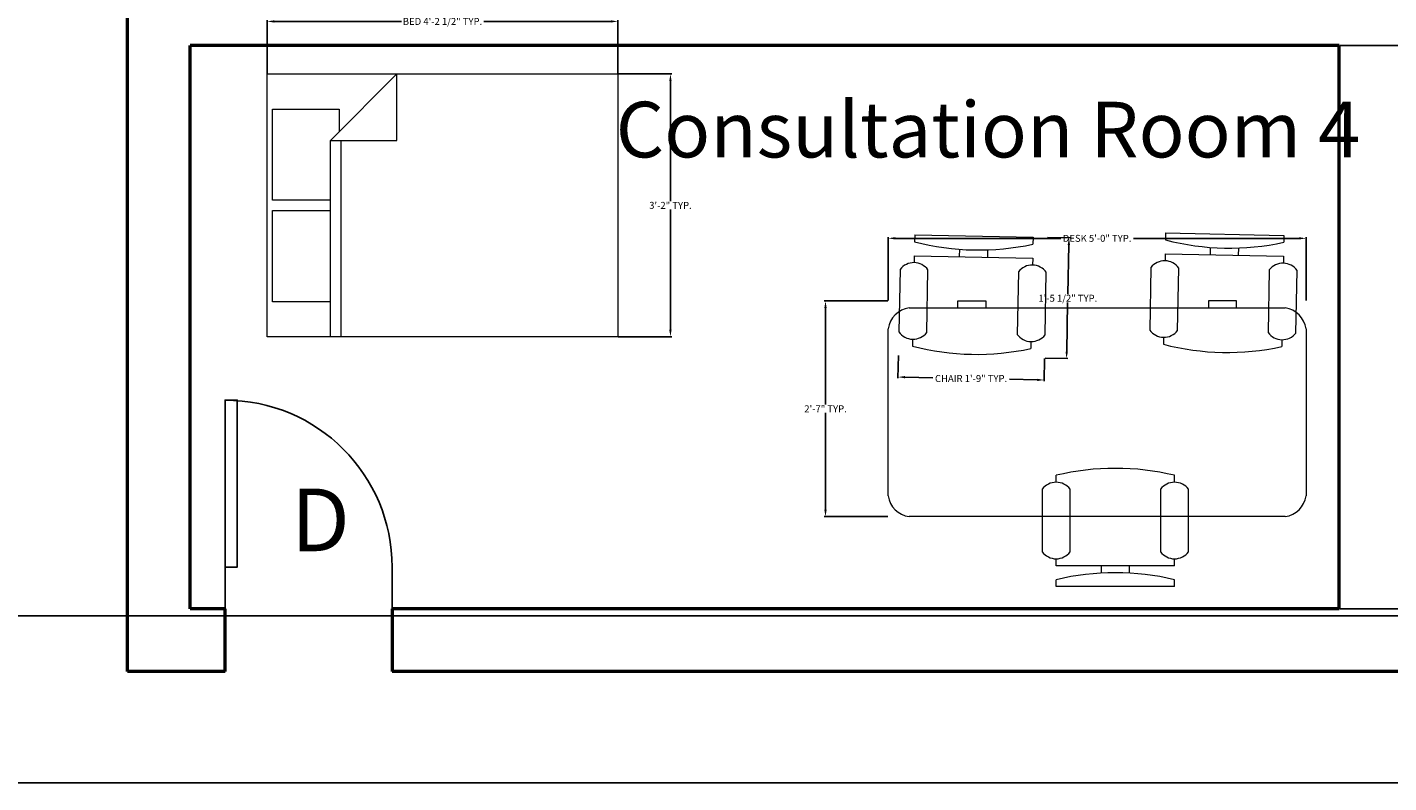
# Model space of a CAD drawing. Units: inches. Extents: x -364 to 705, y -52 to 1250.
# Tile 28 of 34: x 170 to 366, y 806 to 915. Entities that reach past the tile are written whole.
import ezdxf

# ---------------------------------------------------------------- set-up
doc = ezdxf.new("R2010")
doc.units = ezdxf.units.IN
doc.header["$MEASUREMENT"] = 0
for name, color, linetype, lineweight in [('A-ANNO-DIMS', 4, 'Continuous', 18), ('A-ANNO-IDEN', 1, 'Continuous', 18), ('A-AREA-IDEN', 3, 'Continuous', 18), ('A-DOOR', 1, 'Continuous', 25), ('A-FURN', 8, 'Continuous', 18), ('A-WALL', 41, 'Continuous', 50)]:
    doc.layers.add(name, color=color, linetype=linetype, lineweight=lineweight)
doc.styles.get("Standard").update_dxf_attribs({"font": 'arial.ttf'})
doc.dimstyles.get("Standard").update_dxf_attribs({"dimtxt": 1, "dimasz": 1, "dimexe": 0.18, "dimexo": 0.0625, "dimgap": 0.09, "dimtad": 0, "dimtih": 1, "dimtoh": 1, "dimdec": 0, "dimzin": 0, "dimdsep": 46, "dimlunit": 3, "dimtxsty": 'Standard', "dimcen": 0.09, "dimadec": 0, "dimazin": 0, "dimtfac": 1, "dimtdec": 0, "dimtofl": 0, "dimtmove": 0, "dimatfit": 3, "dimfxl": 1, "dimtolj": 1, "dimtzin": 0, "dimarcsym": 0})

# ---------------------------------------------------------------- blocks, each defined once
blk = doc.blocks.new('Chair - Desk')
for p, q in [((-8.5, 0), (-8.5, -1)), ((-8.5, 0), (8.5, 0)), ((8.5, 0), (8.5, -1)), ((-2, -3), (-2, -1.9355)), ((-8.5, -3), (-8.5, -4)), ((-8.5, -3), (8.5, -3)), ((2, -1.9576), (2, -3)), ((8.5, -3), (8.5, -4)), ((-10.5, -5), (-10.5, -14)), ((-6.5, -14), (-6.5, -5)), ((6.5, -5), (6.5, -14)), ((10.5, -14), (10.5, -5)), ((-8.5, -15), (-8.5, -16)), ((8.5, -15), (8.5, -16))]:
    blk.add_line(p, q)
for centre, radius, start, end in [((0, 34.625), 36.625, 256.5803, 283.4197), ((-8.5, -6.5), 2.5, 36.8699, 143.1301), ((8.5, -6.5), 2.5, 36.8699, 143.1301), ((-8.5, -12.5), 2.5, 216.8699, 323.1301), ((8.5, -12.5), 2.5, 216.8699, 323.1301), ((0, 19.625), 36.625, 256.5803, 283.4197)]:
    blk.add_arc(centre, radius, start, end)
blk = doc.blocks.new('Desk - 30 x 60 in.')
for p, q in [((-26.999995, 0), (26.999995, 0)), ((-29.999995, -27), (-29.999995, -3)), ((29.999995, -3), (29.999995, -27)), ((26.999995, -30), (-26.999995, -30)), ((-20.000005, -30), (-20.000005, -31)), ((-20.000005, -31), (-16.000005, -31)), ((-16.000005, -31), (-16.000005, -30)), ((15.999995, -31), (15.999995, -30)), ((19.999995, -31), (15.999995, -31)), ((19.999995, -30), (19.999995, -31))]:
    blk.add_line(p, q)
for centre, start, end in [((-26.499995, -3.5), 98.1301, 171.8699), ((26.499995, -3.5), 8.130102, 81.8699), ((-26.499995, -26.5), 188.1301, 261.8699), ((26.499995, -26.5), 278.1301, 351.8699)]:
    blk.add_arc(centre, 3.535534, start, end)
blk = doc.blocks.new('Bed - Queen')
for p, q in [((0, -80.00003), (0, 0)), ((0, 0), (59.99999, 0)), ((59.99999, 0), (59.99999, -80.00003)), ((7.99999, -1.2), (28.79998, -1.2)), ((7.99999, -14.4), (7.99999, -1.2)), ((28.79998, -1.2), (28.79998, -14.4)), ((31.19999, -1.2), (51.99999, -1.2)), ((31.19999, -14.4), (31.19999, -1.2)), ((51.99999, -1.2), (51.99999, -16.4)), ((0, -14.4), (44.8, -14.4)), ((59.99999, -29.6), (44.8, -14.4)), ((44.8, -14.4), (44.8, -29.6)), ((44.8, -16.8), (0, -16.8)), ((51.99999, -16.4), (46.79936, -16.4)), ((44.8, -29.6), (59.99999, -29.6)), ((59.99999, -80.00003), (0, -80.00003))]:
    blk.add_line(p, q)
blk = doc.blocks.new('*U12')
for p, q in [((0, 0), (0, -6)), ((24, 0), (24, -6))]:
    blk.add_line(p, q)
blk.add_lwpolyline([(0, 0), (0, 24), (1.75, 24), (1.75, 0)], close=True)
blk.add_arc((0, 0), 24, 0, 90)
blk = doc.blocks.new('*D36')
at = {"layer": 'A-ANNO-DIMS', "color": 0, "lineweight": -2, "transparency": 16777216}
for p, q in [((295.27, 867.52), (295.21, 864.25)), ((316.27, 867.09), (316.2, 863.83)), ((296.21, 864.41), (300.21, 864.33)), ((315.21, 864.03), (311.21, 864.11))]:
    blk.add_line(p, q, dxfattribs=at)
at = {"layer": 'A-ANNO-DIMS', "color": 0, "transparency": 16777216}
for points in [[(296.21, 864.58), (296.21, 864.25), (295.21, 864.43)], [(315.21, 864.19), (315.2, 863.86), (316.21, 864.01)]]:
    blk.add_solid(points, dxfattribs=at)
at = {"layer": 'Defpoints', "color": 0, "transparency": 16777216}
for p in [(295.28, 867.58), (316.27, 867.16), (316.21, 864.01)]:
    blk.add_point(p, dxfattribs=at)
at = {"layer": 'A-ANNO-DIMS', "color": 0, "transparency": 16777216, "insert": (305.71, 864.22), "char_height": 1, "attachment_point": 5}
blk.add_mtext('\\A1;CHAIR 1\'-9" TYP.', dxfattribs=at)
blk = doc.blocks.new('*D37')
at = {"layer": 'A-ANNO-DIMS', "color": 0, "lineweight": -2, "transparency": 16777216}
for p, q in [((316.68, 884.49), (319.95, 884.42)), ((319.75, 883.42), (319.61, 876.36)), ((319.44, 868.09), (319.58, 875.15)), ((316.33, 867.16), (319.6, 867.09))]:
    blk.add_line(p, q, dxfattribs=at)
at = {"layer": 'A-ANNO-DIMS', "color": 0, "transparency": 16777216}
for points in [[(319.58, 883.43), (319.92, 883.42), (319.77, 884.42)], [(319.27, 868.1), (319.61, 868.09), (319.42, 867.09)]]:
    blk.add_solid(points, dxfattribs=at)
at = {"layer": 'Defpoints', "color": 0, "transparency": 16777216}
for p in [(316.62, 884.49), (319.77, 884.42), (316.27, 867.16)]:
    blk.add_point(p, dxfattribs=at)
at = {"layer": 'A-ANNO-DIMS', "color": 0, "transparency": 16777216, "insert": (319.6, 875.76), "char_height": 1, "attachment_point": 5}
blk.add_mtext('\\A1;1\'-5 1/2" TYP.', dxfattribs=at)
blk = doc.blocks.new('*D46')
at = {"layer": 'A-ANNO-DIMS', "color": 0, "lineweight": -2, "transparency": 16777216}
for p, q in [((293.81, 875.44), (293.81, 884.55)), ((294.81, 884.37), (318.6, 884.37)), ((352.81, 884.37), (329.02, 884.37)), ((353.81, 875.44), (353.81, 884.55))]:
    blk.add_line(p, q, dxfattribs=at)
at = {"layer": 'A-ANNO-DIMS', "color": 0, "transparency": 16777216}
for points in [[(294.81, 884.54), (294.81, 884.21), (293.81, 884.37)], [(352.81, 884.54), (352.81, 884.21), (353.81, 884.37)]]:
    blk.add_solid(points, dxfattribs=at)
at = {"layer": 'Defpoints', "color": 0, "transparency": 16777216}
for p in [(293.81, 884.37), (293.81, 875.37), (353.81, 875.37)]:
    blk.add_point(p, dxfattribs=at)
at = {"layer": 'A-ANNO-DIMS', "color": 0, "transparency": 16777216, "insert": (323.81, 884.37), "char_height": 1, "attachment_point": 5}
blk.add_mtext('\\A1;DESK 5\'-0" TYP.', dxfattribs=at)
blk = doc.blocks.new('*D47')
at = {"layer": 'A-ANNO-DIMS', "color": 0, "lineweight": -2, "transparency": 16777216}
for p, q in [((293.75, 875.37), (284.63, 875.37)), ((284.81, 874.37), (284.81, 860.47)), ((284.81, 845.37), (284.81, 859.28)), ((293.75, 844.37), (284.63, 844.37))]:
    blk.add_line(p, q, dxfattribs=at)
at = {"layer": 'A-ANNO-DIMS', "color": 0, "transparency": 16777216}
for points in [[(284.64, 874.37), (284.97, 874.37), (284.81, 875.37)], [(284.64, 845.37), (284.97, 845.37), (284.81, 844.37)]]:
    blk.add_solid(points, dxfattribs=at)
at = {"layer": 'Defpoints', "color": 0, "transparency": 16777216}
for p in [(293.81, 875.37), (284.81, 844.37), (293.81, 844.37)]:
    blk.add_point(p, dxfattribs=at)
at = {"layer": 'A-ANNO-DIMS', "color": 0, "transparency": 16777216, "insert": (284.81, 859.87), "char_height": 1, "attachment_point": 5}
blk.add_mtext('\\A1;2\'-7" TYP.', dxfattribs=at)
blk = doc.blocks.new('*D62')
at = {"layer": 'A-ANNO-DIMS', "color": 0, "lineweight": -2, "transparency": 16777216}
for p, q in [((204.64, 908.06), (204.64, 915.73)), ((205.64, 915.55), (223.9, 915.55)), ((253.99, 915.55), (235.72, 915.55)), ((254.99, 908.06), (254.99, 915.73))]:
    blk.add_line(p, q, dxfattribs=at)
at = {"layer": 'A-ANNO-DIMS', "color": 0, "transparency": 16777216}
for points in [[(205.64, 915.71), (205.64, 915.38), (204.64, 915.55)], [(253.99, 915.71), (253.99, 915.38), (254.99, 915.55)]]:
    blk.add_solid(points, dxfattribs=at)
at = {"layer": 'Defpoints', "color": 0, "transparency": 16777216}
for p in [(204.64, 915.55), (204.64, 907.99), (254.99, 907.99)]:
    blk.add_point(p, dxfattribs=at)
at = {"layer": 'A-ANNO-DIMS', "color": 0, "transparency": 16777216, "insert": (229.81, 915.55), "char_height": 1, "attachment_point": 5}
blk.add_mtext('\\A1;BED 4\'-2 1/2" TYP.', dxfattribs=at)
blk = doc.blocks.new('*D63')
at = {"layer": 'A-ANNO-DIMS', "color": 0, "lineweight": -2, "transparency": 16777216}
for p, q in [((255.05, 907.99), (262.72, 907.99)), ((262.54, 906.99), (262.54, 889.71)), ((262.54, 871.23), (262.54, 888.51)), ((255.05, 870.23), (262.72, 870.23))]:
    blk.add_line(p, q, dxfattribs=at)
at = {"layer": 'A-ANNO-DIMS', "color": 0, "transparency": 16777216}
for points in [[(262.37, 906.99), (262.71, 906.99), (262.54, 907.99)], [(262.37, 871.23), (262.71, 871.23), (262.54, 870.23)]]:
    blk.add_solid(points, dxfattribs=at)
at = {"layer": 'Defpoints', "color": 0, "transparency": 16777216}
for p in [(254.99, 907.99), (262.54, 907.99), (254.99, 870.23)]:
    blk.add_point(p, dxfattribs=at)
at = {"layer": 'A-ANNO-DIMS', "color": 0, "transparency": 16777216, "insert": (262.54, 889.11), "char_height": 1, "attachment_point": 5}
blk.add_mtext('\\A1;3\'-2" TYP.', dxfattribs=at)
blk = doc.blocks.new('*D97')
at = {"layer": 'A-ANNO-DIMS', "color": 0, "lineweight": -2, "transparency": 16777216}
for p, q in [((358.64, 912.11), (703.01, 912.11)), ((702.83, 911.11), (702.83, 872.22)), ((702.83, 832.11), (702.83, 871.01)), ((358.64, 831.11), (703.01, 831.11))]:
    blk.add_line(p, q, dxfattribs=at)
at = {"layer": 'A-ANNO-DIMS', "color": 0, "transparency": 16777216}
for points in [[(702.66, 911.11), (703, 911.11), (702.83, 912.11)], [(702.66, 832.11), (703, 832.11), (702.83, 831.11)]]:
    blk.add_solid(points, dxfattribs=at)
at = {"layer": 'Defpoints', "color": 0, "transparency": 16777216}
for p in [(358.58, 912.11), (358.58, 831.11), (702.83, 831.11)]:
    blk.add_point(p, dxfattribs=at)
at = {"layer": 'A-ANNO-DIMS', "color": 0, "transparency": 16777216, "insert": (702.83, 871.61), "char_height": 1, "attachment_point": 5}
blk.add_mtext('\\A1;6\'-9"', dxfattribs=at)
blk = doc.blocks.new('*D105')
at = {"layer": 'A-ANNO-DIMS', "color": 0, "lineweight": -2, "transparency": 16777216}
for p, q in [((148.64, 830.11), (703.01, 830.11)), ((702.83, 829.11), (702.83, 818.72)), ((702.83, 807.11), (702.83, 817.51)), ((148.64, 806.11), (703.01, 806.11))]:
    blk.add_line(p, q, dxfattribs=at)
at = {"layer": 'A-ANNO-DIMS', "color": 0, "transparency": 16777216}
for points in [[(702.66, 829.11), (703, 829.11), (702.83, 830.11)], [(702.66, 807.11), (703, 807.11), (702.83, 806.11)]]:
    blk.add_solid(points, dxfattribs=at)
at = {"layer": 'Defpoints', "color": 0, "transparency": 16777216}
for p in [(148.58, 830.11), (148.58, 806.11), (702.83, 806.11)]:
    blk.add_point(p, dxfattribs=at)
at = {"layer": 'A-ANNO-DIMS', "color": 0, "transparency": 16777216, "insert": (702.83, 818.11), "char_height": 1, "attachment_point": 5}
blk.add_mtext('\\A1;2\'-0"', dxfattribs=at)

msp = doc.modelspace()

# ---------------------------------------------------------------- linework, layer by layer
at = {"layer": 'A-WALL'}
for p, q in [((184.58, 822.11), (184.58, 922.11)), ((193.58, 831.11), (193.58, 912.11)), ((358.58, 912.11), (193.58, 912.11)), ((358.58, 831.11), (358.58, 912.11)), ((198.58, 831.11), (193.58, 831.11)), ((198.58, 822.11), (198.58, 831.11)), ((358.58, 831.11), (222.58, 831.11)), ((222.58, 831.11), (222.58, 822.11)), ((198.58, 822.11), (184.58, 822.11)), ((372.58, 822.11), (222.58, 822.11))]:
    msp.add_line(p, q, dxfattribs=at)

# ---------------------------------------------------------------- block references
at = {"layer": 'A-DOOR'}
msp.add_blockref('*U12', (198.58, 837.11), dxfattribs=at)
at = {"layer": 'A-FURN', "xscale": 0.6293684586277993, "yscale": 0.6293684586277993, "zscale": 0.6293684586277993, "rotation": 90}
msp.add_blockref('Bed - Queen', (204.64, 870.23), dxfattribs=at)
at = {"layer": 'A-FURN'}
for name, p, rotation in [('Chair - Desk', (306.12, 884.7), 358.8399543093714), ('Chair - Desk', (342.14, 884.97), 358.8399543093714), ('Desk - 30 x 60 in.', (323.81, 844.37), 180), ('Chair - Desk', (326.43, 834.31), 180)]:
    msp.add_blockref(name, p, dxfattribs=dict(at, rotation=rotation))

# ---------------------------------------------------------------- texts
at = {"layer": 'A-ANNO-IDEN', "insert": (208.05, 848.4), "char_height": 9, "attachment_point": 1}
msp.add_mtext_dynamic_manual_height_columns('D', width=16.916, gutter_width=1, heights=[0], dxfattribs=at)
at = {"layer": 'A-AREA-IDEN', "insert": (254.68, 904), "char_height": 8, "attachment_point": 1}
msp.add_mtext_dynamic_manual_height_columns('Consultation Room 4', width=124.8937, gutter_width=1, heights=[0], dxfattribs=at)

# ---------------------------------------------------------------- dimensions: what is measured, and where the dimension line sits
at = {"layer": 'A-ANNO-DIMS'}
for base, p1, p2, angle, text, picture, middle in [((204.6375, 915.5467), (254.987, 907.9942), (204.6375, 907.9942), 180, 'BED <> TYP.', '*D62', (229.8123, 915.5467)), ((262.54, 907.99), (254.99, 870.23), (254.99, 907.99), 90, '<> TYP.', '*D63', (262.54, 889.11)), ((293.81, 884.37), (353.81, 875.37), (293.81, 875.37), 180, 'DESK <> TYP.', '*D46', (323.81, 884.37)), ((319.77, 884.42), (316.27, 867.16), (316.62, 884.49), 88.84, '<> TYP.', '*D37', (319.6, 875.76)), ((284.81, 844.37), (293.81, 875.37), (293.81, 844.37), 270, '<> TYP.', '*D47', (284.81, 859.87)), ((316.21, 864.01), (295.28, 867.58), (316.27, 867.16), 358.84, 'CHAIR <> TYP.', '*D36', (305.71, 864.22))]:
    dim = msp.add_linear_dim(base=base, p1=p1, p2=p2, angle=angle, text=text, dimstyle='Standard', override={"dimdec": 1, "dimlfac": 1, "dimrnd": 0, "dimzin": 1, "dimdsep": 46, "dimlunit": 4, "dimfrac": 2}, dxfattribs=at)
    dim.commit()
    dim.dimension.update_dxf_attribs({"geometry": picture, "text_midpoint": middle})
for base, p1, p2, picture, middle in [((702.83, 831.11), (358.58, 912.11), (358.58, 831.11), '*D97', (702.83, 871.61)), ((702.83, 806.11), (148.58, 830.11), (148.58, 806.11), '*D105', (702.83, 818.11))]:
    dim = msp.add_linear_dim(base=base, p1=p1, p2=p2, angle=90, dimstyle='Standard', override={"dimdec": 1, "dimlfac": 1, "dimrnd": 0, "dimzin": 1, "dimdsep": 46, "dimlunit": 4, "dimfrac": 2}, dxfattribs=at)
    dim.commit()
    dim.dimension.update_dxf_attribs({"geometry": picture, "text_midpoint": middle})

doc.saveas('drawing.dxf')
